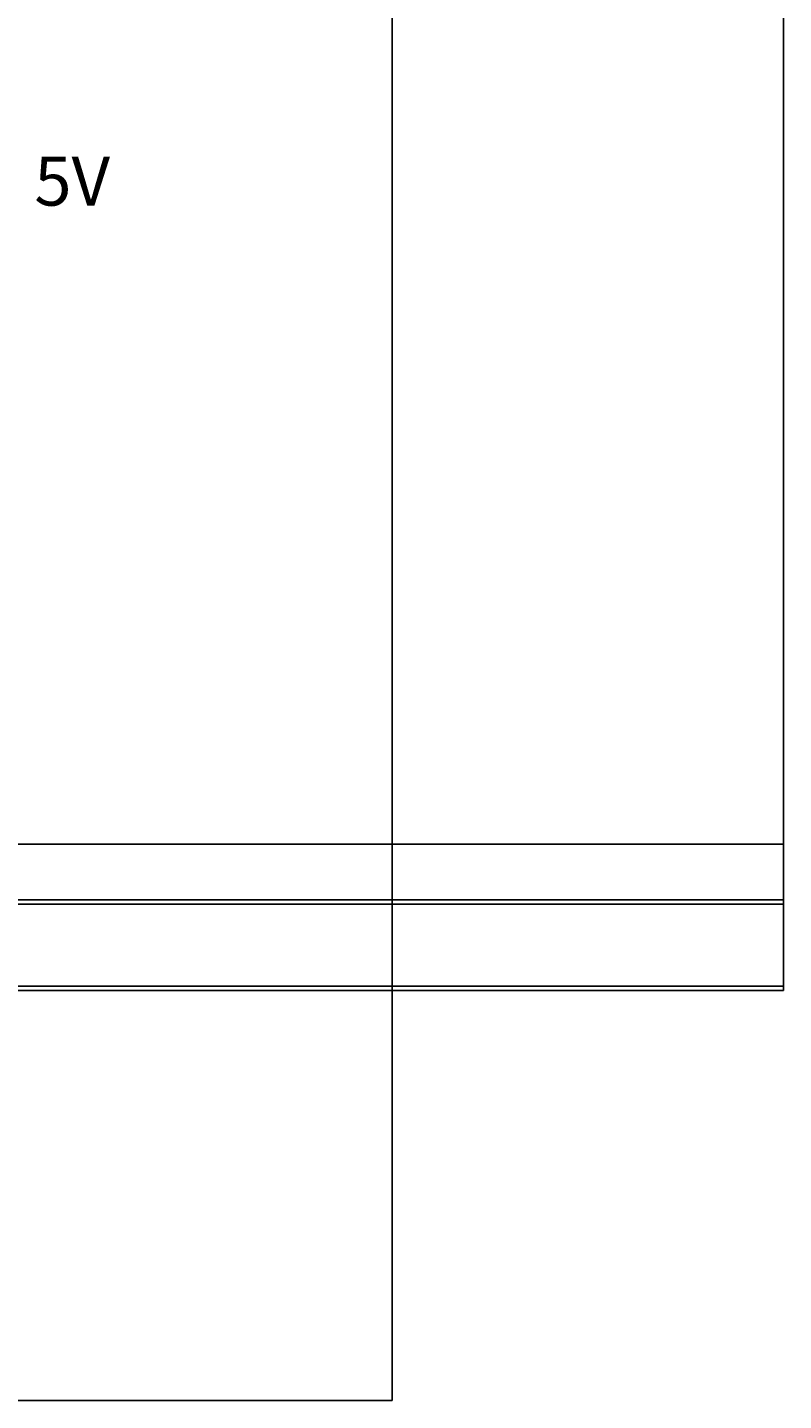
# Model space of a CAD drawing. Units: inches. Extents: x 35362 to 73946, y 43607 to 67532.
# Tile 133 of 134: x 70544 to 73946, y 43607 to 49781. Entities that reach past the tile are written whole.
import ezdxf

# ---------------------------------------------------------------- set-up
doc = ezdxf.new("R2010")
doc.units = ezdxf.units.IN
doc.header["$MEASUREMENT"] = 0
doc.layers.add('A-ANNO-DIMS', color=2, linetype='Continuous', lineweight=18)
doc.layers.add('E-ANNO-TEXT', color=5, linetype='Continuous', lineweight=18)
doc.styles.get("Standard").update_dxf_attribs({"font": 'arial.ttf'})
doc.dimstyles.get("Standard").update_dxf_attribs({"dimtxt": 0.18, "dimasz": 0.18, "dimexe": 0.18, "dimexo": 0.0625, "dimgap": 0.09, "dimtad": 0, "dimtih": 1, "dimtoh": 1, "dimdec": 4, "dimzin": 0, "dimdsep": 46, "dimtxsty": 'Standard', "dimcen": 0.09, "dimadec": 0, "dimazin": 0, "dimtfac": 1, "dimtdec": 4, "dimtofl": 0, "dimtmove": 0, "dimatfit": 3, "dimfxl": 1, "dimtolj": 1, "dimtzin": 0, "dimarcsym": 0})

# ---------------------------------------------------------------- blocks, each defined once
blk = doc.blocks.new('*D6')
at = {"layer": 'A-ANNO-DIMS', "color": 0, "lineweight": -2, "transparency": 16777216}
for p, q in [((72185.645666, 53702.123839), (72185.645666, 43606.678996)), ((69871.496302, 45449.831951), (69871.496302, 43606.678996)), ((69871.67630199999, 43606.858996), (71028.21104539152, 43606.858996)), ((72185.465666, 43606.858996), (71028.93092260844, 43606.858996))]:
    blk.add_line(p, q, dxfattribs=at)
at = {"layer": 'A-ANNO-DIMS', "color": 0, "transparency": 16777216}
for points in [[(69871.67630199999, 43606.888996), (69871.67630199999, 43606.828996), (69871.496302, 43606.858996)], [(72185.465666, 43606.888996), (72185.465666, 43606.828996), (72185.645666, 43606.858996)]]:
    blk.add_solid(points, dxfattribs=at)
at = {"layer": 'Defpoints', "color": 0, "transparency": 16777216}
for p in [(72185.645666, 53702.186339), (69871.496302, 45449.894451), (72185.645666, 43606.858996)]:
    blk.add_point(p, dxfattribs=at)
at = {"layer": 'A-ANNO-DIMS', "color": 0, "transparency": 16777216, "insert": (71028.57098399999, 43606.858996), "char_height": 0.18, "attachment_point": 5}
blk.add_mtext('\\A1;2314', dxfattribs=at)
blk = doc.blocks.new('*D7')
at = {"layer": 'A-ANNO-DIMS', "color": 0, "lineweight": -2, "transparency": 16777216}
for p, q in [((72185.70816600003, 53702.18633900003), (73945.82566600003, 53702.18633900003)), ((73945.64566600005, 53702.00633900003), (73945.64566600005, 49576.22229813781)), ((73945.64566600005, 45450.07445100001), (73945.64566600005, 49575.85849186223)), ((69871.55880200003, 45449.89445100001), (73945.82566600003, 45449.89445100001))]:
    blk.add_line(p, q, dxfattribs=at)
at = {"layer": 'A-ANNO-DIMS', "color": 0, "transparency": 16777216}
for points in [[(73945.61566600006, 53702.00633900003), (73945.67566600005, 53702.00633900003), (73945.64566600005, 53702.18633900003)], [(73945.61566600006, 45450.07445100001), (73945.67566600005, 45450.07445100001), (73945.64566600005, 45449.89445100001)]]:
    blk.add_solid(points, dxfattribs=at)
at = {"layer": 'Defpoints', "color": 0, "transparency": 16777216}
for p in [(72185.64566600003, 53702.18633900003), (73945.64566600005, 53702.18633900003), (69871.49630200001, 45449.89445100001)]:
    blk.add_point(p, dxfattribs=at)
at = {"layer": 'A-ANNO-DIMS', "color": 0, "transparency": 16777216, "insert": (73945.64566600005, 49576.04039499998), "char_height": 0.18, "attachment_point": 5}
blk.add_mtext('\\A1;8252', dxfattribs=at)
blk = doc.blocks.new('*D74')
at = {"layer": 'A-ANNO-DIMS', "color": 0, "lineweight": -2, "transparency": 16777216}
for p, q in [((55181.69646300003, 46108.87757800001), (73945.82566600003, 46108.87757800001)), ((73945.64566600005, 46108.69757800001), (73945.64566600005, 45983.7251866378)), ((73945.64566600005, 45858.38898900001), (73945.64566600005, 45983.36138036223)), ((55181.69646300003, 45858.20898900001), (73945.82566600003, 45858.20898900001))]:
    blk.add_line(p, q, dxfattribs=at)
at = {"layer": 'A-ANNO-DIMS', "color": 0, "transparency": 16777216}
for points in [[(73945.61566600006, 46108.69757800001), (73945.67566600005, 46108.69757800001), (73945.64566600005, 46108.87757800001)], [(73945.61566600006, 45858.38898900001), (73945.67566600005, 45858.38898900001), (73945.64566600005, 45858.20898900001)]]:
    blk.add_solid(points, dxfattribs=at)
at = {"layer": 'Defpoints', "color": 0, "transparency": 16777216}
for p in [(55181.63396300002, 46108.87757800001), (55181.63396300002, 45858.20898900001), (73945.64566600005, 45858.20898900001)]:
    blk.add_point(p, dxfattribs=at)
at = {"layer": 'A-ANNO-DIMS', "color": 0, "transparency": 16777216, "insert": (73945.64566600005, 45983.54328349999), "char_height": 0.18, "attachment_point": 5}
blk.add_mtext('\\A1;250.67', dxfattribs=at)
blk = doc.blocks.new('*D75')
at = {"layer": 'A-ANNO-DIMS', "color": 0, "lineweight": -2, "transparency": 16777216}
for p, q in [((55181.69646300003, 45838.20898900001), (73945.82566600003, 45838.20898900001)), ((73945.64566600005, 45838.02898900001), (73945.64566600005, 45654.23368452933)), ((73945.64566600005, 45470.07445100001), (73945.64566600005, 45653.86975547068)), ((55181.69646300003, 45469.89445100001), (73945.82566600003, 45469.89445100001))]:
    blk.add_line(p, q, dxfattribs=at)
at = {"layer": 'A-ANNO-DIMS', "color": 0, "transparency": 16777216}
for points in [[(73945.61566600006, 45838.02898900001), (73945.67566600005, 45838.02898900001), (73945.64566600005, 45838.20898900001)], [(73945.61566600006, 45470.07445100001), (73945.67566600005, 45470.07445100001), (73945.64566600005, 45469.89445100001)]]:
    blk.add_solid(points, dxfattribs=at)
at = {"layer": 'Defpoints', "color": 0, "transparency": 16777216}
for p in [(55181.63396300002, 45838.20898900001), (55181.63396300002, 45469.89445100001), (73945.64566600005, 45469.89445100001)]:
    blk.add_point(p, dxfattribs=at)
at = {"layer": 'A-ANNO-DIMS', "color": 0, "transparency": 16777216, "insert": (73945.64566600005, 45654.05171999998), "char_height": 0.18, "attachment_point": 5}
blk.add_mtext('\\A1;368.3', dxfattribs=at)

msp = doc.modelspace()

# ---------------------------------------------------------------- texts
at = {"layer": 'E-ANNO-TEXT'}
msp.add_text('5V', height=220.8659825270206, dxfattribs=at).set_placement((70575.37815130001, 48979.47952296854))

# ---------------------------------------------------------------- dimensions: what is measured, and where the dimension line sits
at = {"layer": 'A-ANNO-DIMS'}
dim = msp.add_linear_dim(base=(72185.645666, 43606.858996), p1=(69871.496302, 45449.894451), p2=(72185.645666, 53702.186339), dimstyle='Standard', override={"dimdec": 0, "dimlfac": 1, "dimrnd": 0, "dimzin": 0, "dimdsep": 46, "dimlunit": 2}, dxfattribs=at)
dim.commit()
dim.dimension.update_dxf_attribs({"geometry": '*D6', "text_midpoint": (71028.57098399999, 43606.858996)})
for base, p1, p2, override, picture, middle in [((73945.64566600005, 53702.18633900003), (69871.496302, 45449.894451), (72185.645666, 53702.186339), {"dimdec": 0, "dimlfac": 1, "dimrnd": 0, "dimzin": 0, "dimdsep": 46, "dimlunit": 2}, '*D7', (73945.64566600005, 49576.04039499998)), ((73945.64566600005, 45858.20898900001), (55181.633963, 46108.877578), (55181.633963, 45858.20898899999), {"dimdec": 2, "dimlfac": 1, "dimrnd": 0, "dimzin": 0, "dimdsep": 46, "dimlunit": 2}, '*D74', (73945.64566600005, 45983.54328349999)), ((73945.64566600005, 45469.89445100001), (55181.633963, 45838.20898899999), (55181.633963, 45469.894451), {"dimdec": 1, "dimlfac": 1, "dimrnd": 0, "dimzin": 0, "dimdsep": 46, "dimlunit": 2}, '*D75', (73945.64566600005, 45654.05171999998))]:
    dim = msp.add_linear_dim(base=base, p1=p1, p2=p2, angle=90, dimstyle='Standard', override=override, dxfattribs=at)
    dim.commit()
    dim.dimension.update_dxf_attribs({"geometry": picture, "text_midpoint": middle})

doc.saveas('drawing.dxf')
